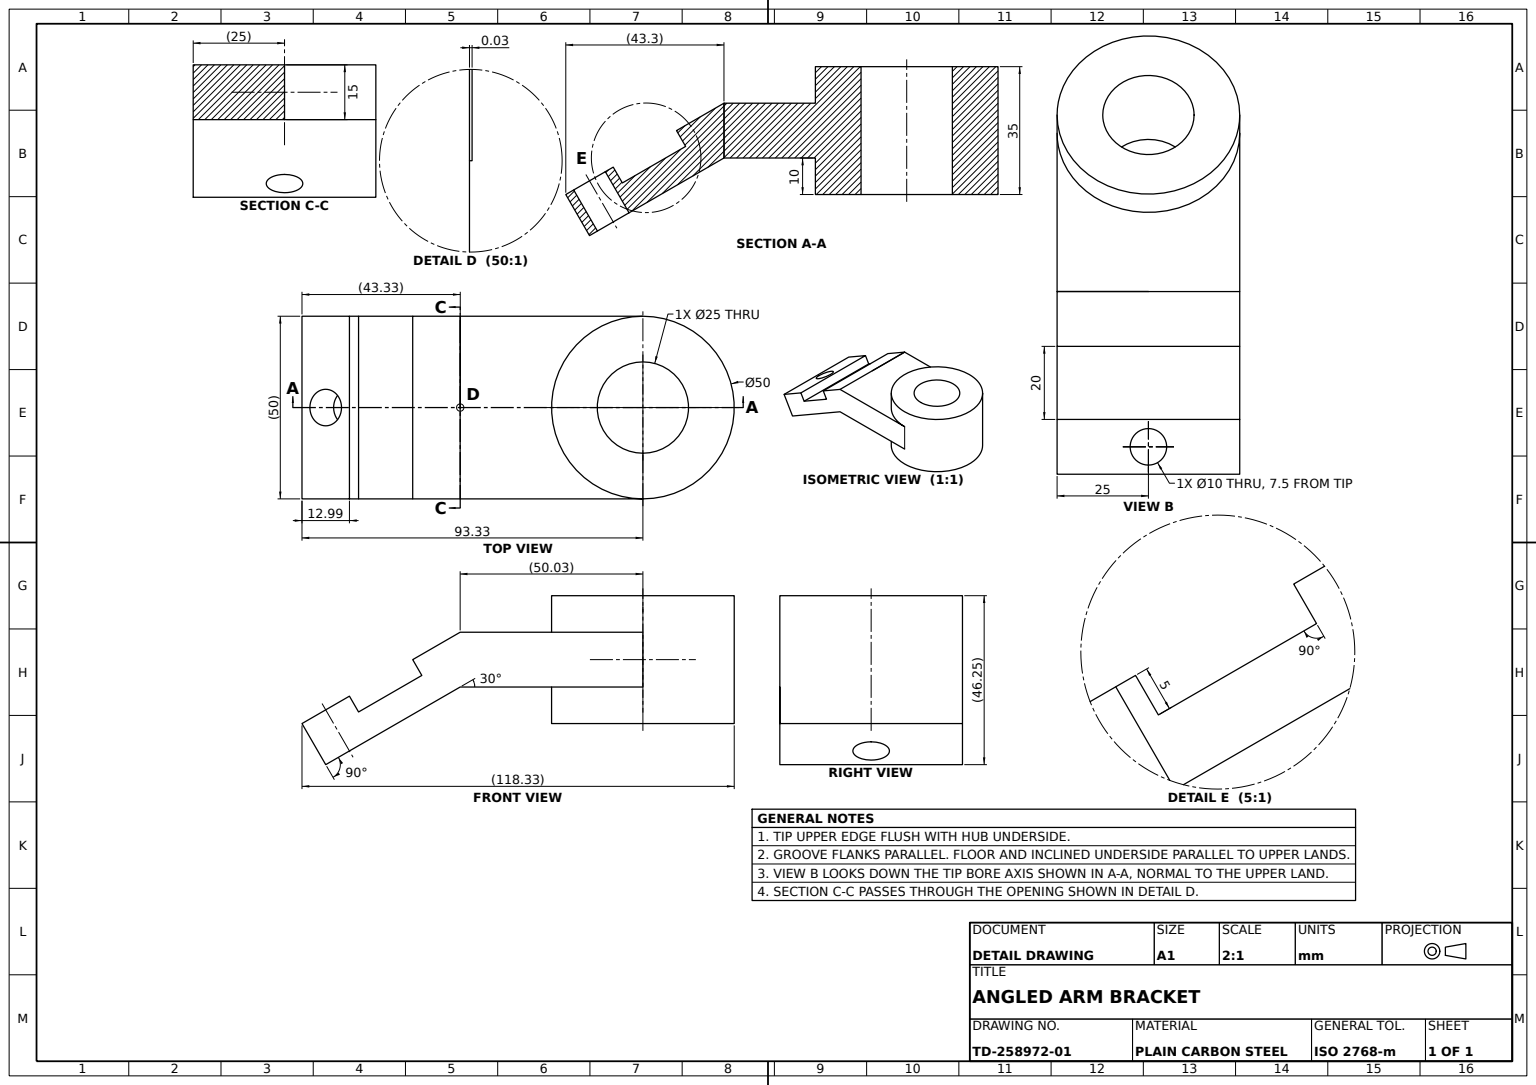
from build123d import *

# Parameters (mm, degrees)
HUB_BASE_25_SKETCH_R       = 12.5
HUB_BASE_25_DEPTH          = 10
HUB_SECTION_1_50_SKETCH_R  = 25
HUB_SECTION_1_50_DEPTH     = 10
HUB_NECK_1_25_SKETCH_R     = 12.5
HUB_NECK_1_25_DEPTH        = 15
HUB_SECTION_2_50_SKETCH_R  = 25
HUB_SECTION_2_50_DEPTH     = 15
HUB_NECK_2_25_SKETCH_R     = 12.5
HUB_NECK_2_25_DEPTH        = 10
HUB_TOP_50_SKETCH_R        = 25
HUB_TOP_50_DEPTH           = 10
ARM_BLOCK_SKETCH_W         = 25
ARM_BLOCK_SKETCH_H         = 15
ARM_BLOCK_DEPTH            = 25
ARM_WEB_PROFILE_SKETCH_W   = 50
ARM_WEB_PROFILE_SKETCH_H   = 25
ARM_WEB_PROFILE_SKETCH_W_2 = 50.02861625
ARM_WEB_DEPTH              = 25
ARM_START                  = -10
ARM_NOTCH_CUT_DEPTH        = 10
NOTCH_FILLER_SKETCH_R      = 25
NOTCH_FILLER_BOSS_DEPTH    = 10
HUB_BORE_25_DEPTH          = 34
HUB_BORE_25_DEPTH_BACK     = 80
HUB_BORE_25_SKETCH_R       = 12.5
DOVETAIL_RAIL_DEPTH        = 50
RAIL_GROOVE_CUT_DEPTH      = 271
RAIL_GROOVE_CUT_DEPTH_BACK = 142
RAIL_HOLE_10_DEPTH         = 179
RAIL_HOLE_10_DEPTH_BACK    = 179
RAIL_HOLE_10_SKETCH_R      = 5


with BuildPart() as part:
    # Hub Base _25 Sketch → Hub Base _25 (new body)
    with BuildSketch(Plane(origin=(0, 0, 0), x_dir=(1, 0, 0), z_dir=(0, 1, 0))):
        with Locations(Location((0, 0, 0), (0, 0, 270))):
            Circle(HUB_BASE_25_SKETCH_R)
    extrude(amount=HUB_BASE_25_DEPTH)

    # Hub Section 1 _50 Sketch → Hub Section 1 _50 (add)
    with BuildSketch(Plane(origin=(0, 10, 0), x_dir=(1, 0, 0), z_dir=(0, 1, 0))):
        with Locations(Location((0, 0, 0), (0, 0, 270))):
            Circle(HUB_SECTION_1_50_SKETCH_R)
    extrude(amount=-HUB_SECTION_1_50_DEPTH)

    # Hub Neck 1 _25 Sketch → Hub Neck 1 _25 (add)
    with BuildSketch(Plane(origin=(0, 10, 0), x_dir=(1, 0, 0), z_dir=(0, 1, 0))):
        with Locations(Location((0, 0, 0), (0, 0, 270))):
            Circle(HUB_NECK_1_25_SKETCH_R)
    extrude(amount=HUB_NECK_1_25_DEPTH)

    # Hub Section 2 _50 Sketch → Hub Section 2 _50 (add)
    with BuildSketch(Plane(origin=(0, 25, 0), x_dir=(1, 0, 0), z_dir=(0, 1, 0))):
        with Locations(Location((0, 0, 0), (0, 0, 270))):
            Circle(HUB_SECTION_2_50_SKETCH_R)
    extrude(amount=-HUB_SECTION_2_50_DEPTH)

    # Hub Neck 2 _25 Sketch → Hub Neck 2 _25 (add)
    with BuildSketch(Plane(origin=(0, 25, 0), x_dir=(1, 0, 0), z_dir=(0, 1, 0))):
        with Locations(Location((0, 0, 0), (0, 0, 270))):
            Circle(HUB_NECK_2_25_SKETCH_R)
    extrude(amount=HUB_NECK_2_25_DEPTH)

    # Hub Top _50 Sketch → Hub Top _50 (add)
    with BuildSketch(Plane(origin=(0, 35, 0), x_dir=(1, 0, 0), z_dir=(0, 1, 0))):
        with Locations(Location((0, 0, 0), (0, 0, 270))):
            Circle(HUB_TOP_50_SKETCH_R)
    extrude(amount=-HUB_TOP_50_DEPTH)



with BuildPart() as body_2:
    # Arm Block Sketch → Arm Block (new, symmetric)
    with BuildSketch(Plane.XY):
        with Locations((-37.5, 17.5)):
            Rectangle(ARM_BLOCK_SKETCH_W, ARM_BLOCK_SKETCH_H)
    extrude(amount=ARM_BLOCK_DEPTH, both=True)


with BuildPart() as part_1:
    add(part.part)

    add(body_2.part)  # Arm Web merges body 2
    # Arm Web Profile Sketch → Arm Web (add)
    with BuildSketch(Plane(origin=(0, 0, 0), x_dir=(1, 0, 0), z_dir=(0, 1, 0))):
        with Locations((-25, 12.5)):
            Rectangle(ARM_WEB_PROFILE_SKETCH_W, ARM_WEB_PROFILE_SKETCH_H)
        with Locations((-25.014308125, -12.5)):
            Rectangle(ARM_WEB_PROFILE_SKETCH_W_2, ARM_WEB_PROFILE_SKETCH_H)
    extrude(amount=ARM_WEB_DEPTH)

    # Arm Notch Sketch → Arm Notch Cut (cut)
    with BuildSketch(Plane.XZ.offset(ARM_START)):
        with BuildLine():
            Line((-2.42391296, 25), (-50.02861625, 25))
            Line((-50.02861625, 25), (-50.02861625, 0))
            Line((-50.02861625, 0), (-50, 0))
            Line((-50, 0), (-50, -25))
            Line((-50, -25), (-2.42391296, -25))
            ThreePointArc((-2.42391296, -25), (-25.117232213, 0), (-2.42391296, 25))
        make_face()
        with BuildLine():
            Line((0, 25), (-2.42391296, 25))
            ThreePointArc((-2.42391296, 25), (-25.117232213, 0), (-2.42391296, -25))
            Line((-2.42391296, -25), (0, -25))
            Line((0, -25), (0, 25))
        make_face()
        with BuildLine():
            Line((0, 25), (0, -25))
            ThreePointArc((0, -25), (25, 0), (0, 25))
        make_face()
    extrude(amount=ARM_NOTCH_CUT_DEPTH, mode=Mode.SUBTRACT)

    # Notch Filler Sketch → Notch Filler Boss (add)
    with BuildSketch(Plane.XZ.offset(-10)):
        with Locations(Location((0, 0, 0), (0, 0, 90))):
            Circle(NOTCH_FILLER_SKETCH_R)
    extrude(amount=NOTCH_FILLER_BOSS_DEPTH)

    # Hub Bore _25 Sketch → Hub Bore _25 (cut, two sides: drawn at the far end of the back side and taken through both)
    with BuildSketch(Plane(origin=(0, 35, 0), x_dir=(1, 0, 0), z_dir=(0, 1, 0)).offset(-HUB_BORE_25_DEPTH_BACK)):
        with Locations(Location((0, 0, 0), (0, 0, 90))):
            Circle(HUB_BORE_25_SKETCH_R)
    extrude(amount=HUB_BORE_25_DEPTH + HUB_BORE_25_DEPTH_BACK, mode=Mode.SUBTRACT)

    # Dovetail Rail Sketch → Dovetail Rail (add)
    with BuildSketch(Plane.XY.offset(25)):
        Polygon((-50.02861625, 10), (-86.834695911, -11.25), (-93.329886439, 0), (-50.02861625, 25), align=None)
    extrude(amount=-DOVETAIL_RAIL_DEPTH)

    # Rail Groove Sketch → Rail Groove Cut (cut, two sides: drawn at the far end of the back side and taken through both)
    with BuildSketch(Plane.XY.offset(25).offset(-RAIL_GROOVE_CUT_DEPTH_BACK)):
        Polygon((-80.339505382, 7.5), (-77.839505382, 3.169872981), (-60.518997307, 13.169872981), (-63.018997307, 17.5), align=None)
    extrude(amount=RAIL_GROOVE_CUT_DEPTH + RAIL_GROOVE_CUT_DEPTH_BACK, mode=Mode.SUBTRACT)

    # Rail Hole _10 Sketch → Rail Hole _10 (cut, two sides: drawn at the far end of the back side and taken through both)
    with BuildSketch(Plane(origin=(-23.33247161, 40.413026294, 0), x_dir=(0.8660254037844379, 0.5000000000000013, 0), z_dir=(-0.5000000000000013, 0.8660254037844379, 0)).offset(-RAIL_HOLE_10_DEPTH_BACK)):
        with Locations((-73.326052589, 0)):
            Circle(RAIL_HOLE_10_SKETCH_R)
    extrude(amount=RAIL_HOLE_10_DEPTH + RAIL_HOLE_10_DEPTH_BACK, mode=Mode.SUBTRACT)


solid = part_1.part
